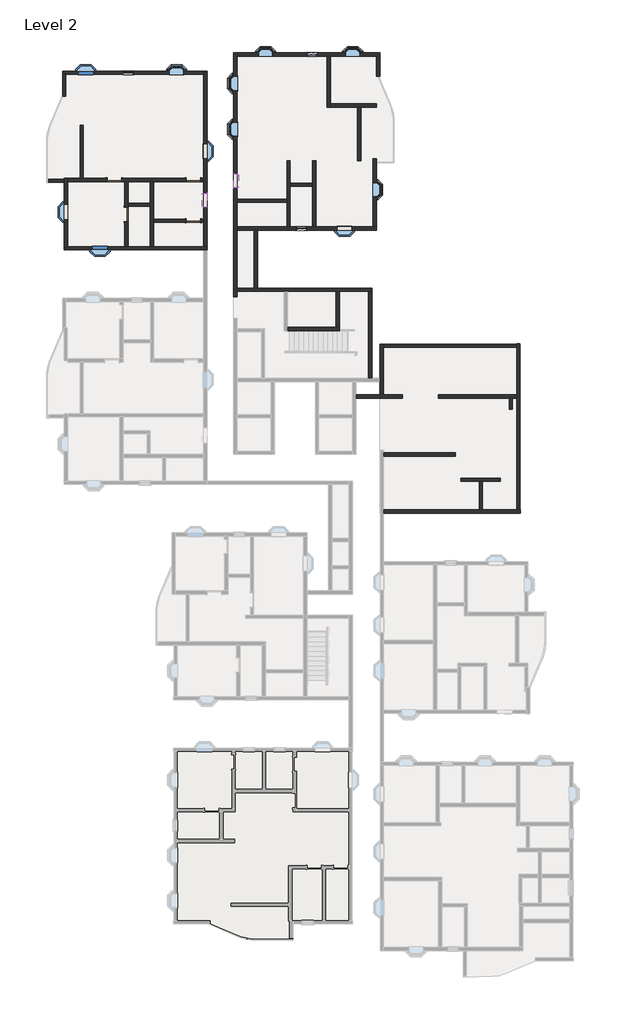
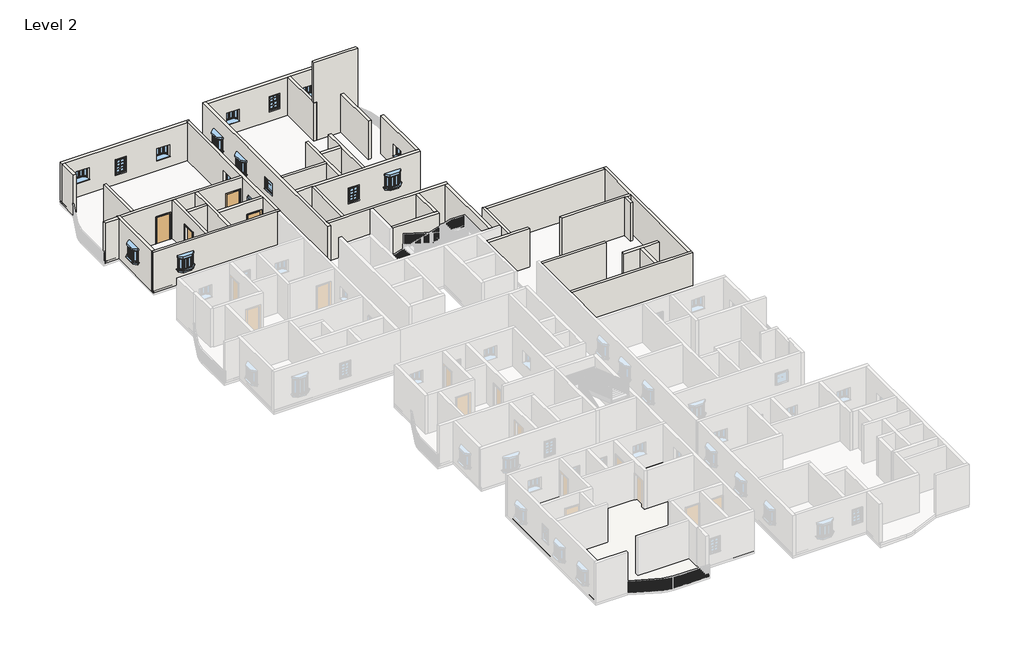
# One storey, part 4 of 14: 40 walls, 16 windows, 4 doors, 1 roof.
"""IFC4 building model written with IfcOpenShell, lengths in millimetres."""

from ifc_helpers import new_model, si_unit, point, frame, frame_2d, origin, place, context, project, spatial, polyline, circle_curve, trimmed, segment, composite_curve, outline, extrude, faceted_brep, transform, mapped, element, save
from components import door_719f80de, window_910x910mm_67ef725a, window_8debb0fa, windows_sgl_w_glazing_bars_910x910mm_256712d0

model = new_model("IFC4")

# Units and contexts
model_context = context("Model", 3, world=origin())
ifc_project = project(units=[si_unit("LENGTHUNIT", "METRE", prefix="MILLI")], contexts=[model_context])

# Site, building, storey
site = spatial("IfcSite", under=ifc_project)
building = spatial("IfcBuilding", under=site)
storey = spatial("IfcBuildingStorey", under=building, Name="Level 2", Elevation=3048.0)

# Doors
placement = place(None, origin())
door_shape = door_719f80de(model_context)
element("IfcDoor", 1, ObjectType="Single-Flush : 36\" x 84\"", at=placement, inside=storey, context=model_context, shape_type="MappedRepresentation", body=[
    mapped(door_shape, transform((-16068.1391351, 22048.4083494, 3048.0), x_axis=(1.0, 0.0, 0.0), y_axis=(0.0, 1.0, 0.0), z_axis=(0.0, 0.0, 1.0))),
])
element("IfcDoor", 2, ObjectType="Single-Flush : 36\" x 84\"", at=placement, inside=storey, context=model_context, shape_type="MappedRepresentation", body=[
    mapped(door_shape, transform((-15306.1391351, 19864.0083494, 3048.0), x_axis=(0.0, 1.0, 0.0), y_axis=(-1.0, 0.0, 0.0), z_axis=(0.0, 0.0, 1.0))),
])
element("IfcDoor", 3, ObjectType="Single-Flush : 36\" x 84\"", at=placement, inside=storey, context=model_context, shape_type="MappedRepresentation", body=[
    mapped(door_shape, transform((-11057.9891351, 19470.3083494, 3048.0), x_axis=(1.0, 0.0, 0.0), y_axis=(0.0, 1.0, 0.0), z_axis=(0.0, 0.0, 1.0))),
])
element("IfcDoor", 4, ObjectType="Single-Flush : 36\" x 84\"", at=placement, inside=storey, context=model_context, shape_type="MappedRepresentation", body=[
    mapped(door_shape, transform((-11057.9891351, 22048.4083494, 3048.0), x_axis=(1.0, 0.0, 0.0), y_axis=(0.0, 1.0, 0.0), z_axis=(0.0, 0.0, 1.0))),
])

# Roof
element("IfcRoof", 5, ObjectType="Generic - 12\"", at=placement, inside=storey, context=model_context, shape_type="SweptSolid", body=[
    extrude(outline(composite_curve([segment(polyline([(-10024.8708389, -25100.3416506), (-12290.487215, -25100.3416506), (-12290.487215, -13962.4416506), (-986.8891351, -13962.4416506), (-986.8891351, -25100.3416506), (-4746.0891351, -25100.3416506), (-4746.0891351, -26090.9416506), (-7315.6413127, -26090.9416506)]), True, "CONTINUOUS"), segment(trimmed(circle_curve(frame_2d((-7315.6413127, -24160.5416506)), 1930.4), [point((-7315.6413127, -26090.9416506))], [point((-8075.5356374, -25935.0851906))], False, "CARTESIAN"), True, "CONTINUOUS"), segment(polyline([(-8075.5356374, -25935.0851906), (-10024.8708389, -25100.3416506)]), True, "CONTINUOUS")], self_intersect=False)), frame((0.0, 0.0, 3048.0), z_axis=(0.0, 0.0, 1.0), x_axis=(1.0, 0.0, 0.0)), (0.0, 0.0, 1.0), 152.4),
])

# Walls
element("IfcWall", 6, ObjectType="4.5\" p", at=placement, inside=storey, context=model_context, shape_type="Brep", body=[
    faceted_brep([(-10600.7891351, 21946.8083494, 5181.6), (-10600.7891351, 21946.8083494, 3048.0), (-10397.5891351, 21946.8083494, 3048.0), (-10397.5891351, 21946.8083494, 6096.0), (-13578.9391351, 21946.8083494, 6096.0), (-13782.1391351, 21946.8083494, 6096.0), (-15204.5391351, 21946.8083494, 6096.0), (-15407.7391351, 21946.8083494, 6096.0), (-19033.5891351, 21946.8083494, 6096.0), (-19033.5891351, 21946.8083494, 3048.0), (-16525.3391351, 21946.8083494, 3048.0), (-16525.3391351, 21946.8083494, 5181.6), (-15610.9391351, 21946.8083494, 5181.6), (-15610.9391351, 21946.8083494, 3048.0), (-15407.7391351, 21946.8083494, 3048.0), (-15204.5391351, 21946.8083494, 3048.0), (-13782.1391351, 21946.8083494, 3048.0), (-13578.9391351, 21946.8083494, 3048.0), (-11515.1891351, 21946.8083494, 3048.0), (-11515.1891351, 21946.8083494, 5181.6), (-10397.5891351, 22150.0083494, 3048.0), (-10600.7891351, 22150.0083494, 3048.0), (-10600.7891351, 22150.0083494, 5181.6), (-11515.1891351, 22150.0083494, 5181.6), (-11515.1891351, 22150.0083494, 3048.0), (-15610.9391351, 22150.0083494, 3048.0), (-15610.9391351, 22150.0083494, 5181.6), (-16525.3391351, 22150.0083494, 5181.6), (-16525.3391351, 22150.0083494, 3048.0), (-18042.9891351, 22150.0083494, 3048.0), (-18246.1891351, 22150.0083494, 3048.0), (-19033.5891351, 22150.0083494, 3048.0), (-19033.5891351, 22150.0083494, 6096.0), (-18246.1891351, 22150.0083494, 6096.0), (-18042.9891351, 22150.0083494, 6096.0), (-10397.5891351, 22150.0083494, 6096.0)], [[[0, 1, 2, 3, 4, 5, 6, 7, 8, 9, 10, 11, 12, 13, 14, 15, 16, 17, 18, 19]], [[20, 21, 22, 23, 24, 25, 26, 27, 28, 29, 30, 31, 32, 33, 34, 35]], [[10, 9, 31, 30, 29, 28]], [[2, 1, 21, 20]], [[18, 17, 16, 15, 14, 13, 25, 24]], [[8, 7, 6, 5, 4, 3, 35, 34, 33, 32]], [[9, 8, 32, 31]], [[3, 2, 20, 35]], [[26, 25, 13, 12]], [[27, 26, 12, 11]], [[28, 27, 11, 10]], [[22, 21, 1, 0]], [[23, 22, 0, 19]], [[24, 23, 19, 18]]]),
])
element("IfcWall", 7, ObjectType="4.5\" p", at=placement, inside=storey, context=model_context, shape_type="Brep", body=[
    faceted_brep([(-15407.7391351, 21946.8083494, 3048.0), (-15407.7391351, 20321.2083494, 3048.0), (-15407.7391351, 20321.2083494, 5181.6), (-15407.7391351, 19406.8083494, 5181.6), (-15407.7391351, 19406.8083494, 3048.0), (-15407.7391351, 17812.9583494, 3048.0), (-15407.7391351, 17812.9583494, 6096.0), (-15407.7391351, 21946.8083494, 6096.0), (-15204.5391351, 20321.2083494, 5181.6), (-15204.5391351, 20321.2083494, 3048.0), (-15204.5391351, 20372.0083494, 3048.0), (-15204.5391351, 20575.2083494, 3048.0), (-15204.5391351, 21946.8083494, 3048.0), (-15204.5391351, 21946.8083494, 6096.0), (-15204.5391351, 20575.2083494, 6096.0), (-15204.5391351, 20372.0083494, 6096.0), (-15204.5391351, 17812.9583494, 6096.0), (-15204.5391351, 17812.9583494, 3048.0), (-15204.5391351, 19406.8083494, 3048.0), (-15204.5391351, 19406.8083494, 5181.6)], [[[0, 1, 2, 3, 4, 5, 6, 7]], [[8, 9, 10, 11, 12, 13, 14, 15, 16, 17, 18, 19]], [[18, 17, 5, 4]], [[12, 11, 10, 9, 1, 0]], [[7, 6, 16, 15, 14, 13]], [[6, 5, 17, 16]], [[0, 7, 13, 12]], [[2, 1, 9, 8]], [[3, 2, 8, 19]], [[4, 3, 19, 18]]]),
])
element("IfcWall", 8, ObjectType="4.5\" p", at=placement, inside=storey, context=model_context, shape_type="Brep", body=[
    faceted_brep([(-13782.1391351, 21946.8083494, 3048.0), (-13782.1391351, 20575.2083494, 3048.0), (-13782.1391351, 20372.0083494, 3048.0), (-13782.1391351, 17812.9583494, 3048.0), (-13782.1391351, 17812.9583494, 6096.0), (-13782.1391351, 20372.0083494, 6096.0), (-13782.1391351, 20575.2083494, 6096.0), (-13782.1391351, 21946.8083494, 6096.0), (-13578.9391351, 21946.8083494, 3048.0), (-13578.9391351, 21946.8083494, 6096.0), (-13578.9391351, 19571.9083494, 6096.0), (-13578.9391351, 19368.7083494, 6096.0), (-13578.9391351, 17812.9583494, 6096.0), (-13578.9391351, 17812.9583494, 3048.0), (-13578.9391351, 19368.7083494, 3048.0), (-13578.9391351, 19571.9083494, 3048.0)], [[[0, 1, 2, 3, 4, 5, 6, 7]], [[8, 9, 10, 11, 12, 13, 14, 15]], [[3, 2, 1, 0, 8, 15, 14, 13]], [[7, 6, 5, 4, 12, 11, 10, 9]], [[4, 3, 13, 12]], [[0, 7, 9, 8]]]),
])
element("IfcWall", 9, ObjectType="4.5\" p", at=placement, inside=storey, context=model_context, shape_type="SweptSolid", body=[
    extrude(outline(polyline([(-13782.1391351, 20372.0083494), (-15204.5391351, 20372.0083494), (-15204.5391351, 20575.2083494), (-13782.1391351, 20575.2083494), (-13782.1391351, 20372.0083494)])), frame((0.0, 0.0, 3048.0), z_axis=(0.0, 0.0, 1.0), x_axis=(1.0, 0.0, 0.0)), (0.0, 0.0, 1.0), 3048.0),
])
element("IfcWall", 10, ObjectType="4.5\" p", at=placement, inside=storey, context=model_context, shape_type="SweptSolid", body=[
    extrude(outline(polyline([(5181.6, -10600.7891351), (3048.0, -10600.7891351), (3048.0, -10397.5891351), (6096.0, -10397.5891351), (6096.0, -13578.9391351), (3048.0, -13578.9391351), (3048.0, -11515.1891351), (5181.6, -11515.1891351), (5181.6, -10600.7891351)])), frame((0.0, 19368.7083494, 0.0), z_axis=(0.0, 1.0, 0.0), x_axis=(0.0, 0.0, 1.0)), (0.0, 0.0, 1.0), 203.2),
])
element("IfcWall", 11, ObjectType="4.5\" p", at=placement, inside=storey, context=model_context, shape_type="SweptSolid", body=[
    extrude(outline(polyline([(-18246.1891351, 22150.0083494), (-18246.1891351, 25515.5083494), (-18042.9891351, 25515.5083494), (-18042.9891351, 22150.0083494), (-18246.1891351, 22150.0083494)])), frame((0.0, 0.0, 3048.0), z_axis=(0.0, 0.0, 1.0), x_axis=(1.0, 0.0, 0.0)), (0.0, 0.0, 1.0), 3048.0),
])
element("IfcWall", 12, ObjectType="4.5\" p", at=placement, inside=storey, context=model_context, shape_type="SweptSolid", body=[
    extrude(outline(polyline([(-6993.9891351, 18875.1215905), (-6993.9891351, 15192.1215905), (-7197.1891351, 15192.1215905), (-7197.1891351, 18875.1215905), (-6993.9891351, 18875.1215905)])), frame((0.0, 0.0, 3048.0), z_axis=(0.0, 0.0, 1.0), x_axis=(1.0, 0.0, 0.0)), (0.0, 0.0, 1.0), 3048.0),
])
element("IfcWall", 13, ObjectType="4.5\" p", at=placement, inside=storey, context=model_context, shape_type="Brep", body=[
    faceted_brep([(-8289.3891351, 18875.1215905, 3048.0), (-7197.1891351, 18875.1215905, 3048.0), (-6993.9891351, 18875.1215905, 3048.0), (562.5108649, 18875.1215905, 3048.0), (562.5108649, 18875.1215905, 6096.0), (-6993.9891351, 18875.1215905, 6096.0), (-7197.1891351, 18875.1215905, 6096.0), (-8289.3891351, 18875.1215905, 6096.0), (-1017.6641351, 18875.1215905, 5158.0), (-1017.6641351, 18875.1215905, 4248.0), (-1927.6641351, 18875.1215905, 4248.0), (-1927.6641351, 18875.1215905, 5158.0), (-3876.1391351, 18875.1215905, 5029.2), (-3876.1391351, 18875.1215905, 3962.4), (-4536.5391351, 18875.1215905, 3962.4), (-4536.5391351, 18875.1215905, 5029.2), (-8289.3891351, 19078.3215905, 3048.0), (-8289.3891351, 19078.3215905, 6096.0), (-5120.7391351, 19078.3215905, 6096.0), (-4917.5391351, 19078.3215905, 6096.0), (-3495.1391351, 19078.3215905, 6096.0), (-3291.9391351, 19078.3215905, 6096.0), (346.6108649, 19078.3215905, 6096.0), (549.8108649, 19078.3215905, 6096.0), (562.5108649, 19078.3215905, 6096.0), (562.5108649, 19078.3215905, 3048.0), (549.8108649, 19078.3215905, 3048.0), (346.6108649, 19078.3215905, 3048.0), (-3291.9391351, 19078.3215905, 3048.0), (-3495.1391351, 19078.3215905, 3048.0), (-4917.5391351, 19078.3215905, 3048.0), (-5120.7391351, 19078.3215905, 3048.0), (-1017.6641351, 19078.3215905, 5158.0), (-1927.6641351, 19078.3215905, 5158.0), (-1927.6641351, 19078.3215905, 4248.0), (-1017.6641351, 19078.3215905, 4248.0), (-3876.1391351, 19078.3215905, 5029.2), (-4536.5391351, 19078.3215905, 5029.2), (-4536.5391351, 19078.3215905, 3962.4), (-3876.1391351, 19078.3215905, 3962.4)], [[[0, 1, 2, 3, 4, 5, 6, 7], [8, 9, 10, 11], [12, 13, 14, 15]], [[16, 17, 18, 19, 20, 21, 22, 23, 24, 25, 26, 27, 28, 29, 30, 31], [32, 33, 34, 35], [36, 37, 38, 39]], [[3, 2, 1, 0, 16, 31, 30, 29, 28, 27, 26, 25]], [[4, 3, 25, 24]], [[7, 6, 5, 4, 24, 23, 22, 21, 20, 19, 18, 17]], [[0, 7, 17, 16]], [[9, 8, 32, 35]], [[10, 9, 35, 34]], [[11, 10, 34, 33]], [[8, 11, 33, 32]], [[13, 12, 36, 39]], [[14, 13, 39, 38]], [[15, 14, 38, 37]], [[12, 15, 37, 36]]]),
])
element("IfcWall", 14, ObjectType="4.5\" p", at=placement, inside=storey, context=model_context, shape_type="SweptSolid", body=[
    extrude(outline(polyline([(19078.3215905, 3048.0), (19078.3215905, 6096.0), (23396.3215905, 6096.0), (23396.3215905, 3048.0), (19078.3215905, 3048.0)]), holes=[polyline([(21882.8215905, 4872.4), (20972.8215905, 4872.4), (20972.8215905, 3962.4), (21882.8215905, 3962.4), (21882.8215905, 4872.4)])]), frame((346.6108649, 0.0, 0.0), z_axis=(1.0, 0.0, 0.0), x_axis=(0.0, 1.0, 0.0)), (0.0, 0.0, 1.0), 203.2),
])
element("IfcWall", 15, ObjectType="4.5\" p", at=placement, inside=storey, context=model_context, shape_type="SweptSolid", body=[
    extrude(outline(polyline([(-5120.7391351, 20634.0715905), (-8289.3891351, 20634.0715905), (-8289.3891351, 20837.2715905), (-5120.7391351, 20837.2715905), (-5120.7391351, 20634.0715905)])), frame((0.0, 0.0, 3048.0), z_axis=(0.0, 0.0, 1.0), x_axis=(1.0, 0.0, 0.0)), (0.0, 0.0, 1.0), 3048.0),
])
element("IfcWall", 16, ObjectType="4.5\" p", at=placement, inside=storey, context=model_context, shape_type="Brep", body=[
    faceted_brep([(-5120.7391351, 23256.6215905, 3048.0), (-5120.7391351, 20837.2715905, 3048.0), (-5120.7391351, 20634.0715905, 3048.0), (-5120.7391351, 19078.3215905, 3048.0), (-5120.7391351, 19078.3215905, 6096.0), (-5120.7391351, 20634.0715905, 6096.0), (-5120.7391351, 20837.2715905, 6096.0), (-5120.7391351, 23256.6215905, 6096.0), (-4917.5391351, 23256.6215905, 3048.0), (-4917.5391351, 23256.6215905, 6096.0), (-4917.5391351, 21853.2715905, 6096.0), (-4917.5391351, 21650.0715905, 6096.0), (-4917.5391351, 19078.3215905, 6096.0), (-4917.5391351, 19078.3215905, 3048.0), (-4917.5391351, 21650.0715905, 3048.0), (-4917.5391351, 21853.2715905, 3048.0)], [[[0, 1, 2, 3, 4, 5, 6, 7]], [[8, 9, 10, 11, 12, 13, 14, 15]], [[3, 2, 1, 0, 8, 15, 14, 13]], [[7, 6, 5, 4, 12, 11, 10, 9]], [[0, 7, 9, 8]], [[4, 3, 13, 12]]]),
])
element("IfcWall", 17, ObjectType="4.5\" p", at=placement, inside=storey, context=model_context, shape_type="Brep", body=[
    faceted_brep([(-3495.1391351, 23256.6215905, 3048.0), (-3495.1391351, 21853.2715905, 3048.0), (-3495.1391351, 21650.0715905, 3048.0), (-3495.1391351, 19078.3215905, 3048.0), (-3495.1391351, 19078.3215905, 6096.0), (-3495.1391351, 21650.0715905, 6096.0), (-3495.1391351, 21853.2715905, 6096.0), (-3495.1391351, 23256.6215905, 6096.0), (-3291.9391351, 23256.6215905, 3048.0), (-3291.9391351, 23256.6215905, 6096.0), (-3291.9391351, 19078.3215905, 6096.0), (-3291.9391351, 19078.3215905, 3048.0)], [[[0, 1, 2, 3, 4, 5, 6, 7]], [[8, 9, 10, 11]], [[3, 2, 1, 0, 8, 11]], [[7, 6, 5, 4, 10, 9]], [[0, 7, 9, 8]], [[4, 3, 11, 10]]]),
])
element("IfcWall", 18, ObjectType="4.5\" p", at=placement, inside=storey, context=model_context, shape_type="SweptSolid", body=[
    extrude(outline(polyline([(-3495.1391351, 21650.0715905), (-4917.5391351, 21650.0715905), (-4917.5391351, 21853.2715905), (-3495.1391351, 21853.2715905), (-3495.1391351, 21650.0715905)])), frame((0.0, 0.0, 3048.0), z_axis=(0.0, 0.0, 1.0), x_axis=(1.0, 0.0, 0.0)), (0.0, 0.0, 1.0), 3048.0),
])
element("IfcWall", 19, ObjectType="4.5\" p", at=placement, inside=storey, context=model_context, shape_type="SweptSolid", body=[
    extrude(outline(polyline([(-1799.6891351, 14988.9215905), (-1799.6891351, 12709.2715905), (-2002.8891351, 12709.2715905), (-2002.8891351, 14988.9215905), (-1799.6891351, 14988.9215905)])), frame((0.0, 0.0, 3048.0), z_axis=(0.0, 0.0, 1.0), x_axis=(1.0, 0.0, 0.0)), (0.0, 0.0, 1.0), 3048.0),
])
element("IfcWall", 20, ObjectType="4.5\" p", at=placement, inside=storey, context=model_context, shape_type="Brep", body=[
    faceted_brep([(-5095.3391351, 12506.0715905, 3048.0), (-1786.9891351, 12506.0715905, 3048.0), (-1786.9891351, 12506.0715905, 6096.0), (-5095.3391351, 12506.0715905, 6096.0), (-5095.3391351, 12709.2715905, 3048.0), (-5095.3391351, 12709.2715905, 6096.0), (-2002.8891351, 12709.2715905, 6096.0), (-1799.6891351, 12709.2715905, 6096.0), (-1786.9891351, 12709.2715905, 6096.0), (-1786.9891351, 12709.2715905, 3048.0), (-1799.6891351, 12709.2715905, 3048.0), (-2002.8891351, 12709.2715905, 3048.0)], [[[0, 1, 2, 3]], [[4, 5, 6, 7, 8, 9, 10, 11]], [[1, 0, 4, 11, 10, 9]], [[2, 1, 9, 8]], [[3, 2, 8, 7, 6, 5]], [[0, 3, 5, 4]]]),
])
element("IfcWall", 21, ObjectType="4.5\" p", at=placement, inside=storey, context=model_context, shape_type="Brep", body=[
    faceted_brep([(-745.5891351, 8223.6457306, 3048.0), (2209.4205024, 8223.6457306, 3048.0), (2209.4205024, 8223.6457306, 6096.0), (-745.5891351, 8223.6457306, 6096.0), (-745.5891351, 8426.8457306, 3048.0), (-745.5891351, 8426.8457306, 6096.0), (793.5880523, 8426.8457306, 6096.0), (996.7880523, 8426.8457306, 6096.0), (2209.4205024, 8426.8457306, 6096.0), (2209.4205024, 8426.8457306, 3048.0), (996.7880523, 8426.8457306, 3048.0), (793.5880523, 8426.8457306, 3048.0)], [[[0, 1, 2, 3]], [[4, 5, 6, 7, 8, 9, 10, 11]], [[1, 0, 4, 11, 10, 9]], [[2, 1, 9, 8]], [[3, 2, 8, 7, 6, 5]], [[0, 3, 5, 4]]]),
])
element("IfcWall", 22, ObjectType="4.5\" p", at=placement, inside=storey, context=model_context, shape_type="Brep", body=[
    faceted_brep([(996.7880523, 8426.8457306, 3048.0), (996.7880523, 11443.0957306, 3048.0), (996.7880523, 11646.2957306, 3048.0), (996.7880523, 11646.2957306, 6096.0), (996.7880523, 11443.0957306, 6096.0), (996.7880523, 8426.8457306, 6096.0), (793.5880523, 8426.8457306, 3048.0), (793.5880523, 8426.8457306, 6096.0), (793.5880523, 9275.2949943, 6096.0), (793.5880523, 9478.4949943, 6096.0), (793.5880523, 11646.2957306, 6096.0), (793.5880523, 11646.2957306, 3048.0), (793.5880523, 9478.4949943, 3048.0), (793.5880523, 9275.2949943, 3048.0)], [[[0, 1, 2, 3, 4, 5]], [[6, 7, 8, 9, 10, 11, 12, 13]], [[2, 1, 0, 6, 13, 12, 11]], [[5, 4, 3, 10, 9, 8, 7]], [[0, 5, 7, 6]], [[3, 2, 11, 10]]]),
])
element("IfcWall", 23, ObjectType="4.5\" p", at=placement, inside=storey, context=model_context, shape_type="Brep", body=[
    faceted_brep([(9461.3380523, 8426.8457306, 3048.0), (4492.3034266, 8426.8457306, 3048.0), (4492.3034266, 8426.8457306, 6096.0), (9461.3380523, 8426.8457306, 6096.0), (9461.3380523, 8223.6457306, 3048.0), (9461.3380523, 8223.6457306, 6096.0), (9181.9380523, 8223.6457306, 6096.0), (8978.7380523, 8223.6457306, 6096.0), (4492.3034266, 8223.6457306, 6096.0), (4492.3034266, 8223.6457306, 3048.0), (8978.7380523, 8223.6457306, 3048.0), (9181.9380523, 8223.6457306, 3048.0)], [[[0, 1, 2, 3]], [[4, 5, 6, 7, 8, 9, 10, 11]], [[1, 0, 4, 11, 10, 9]], [[2, 1, 9, 8]], [[3, 2, 8, 7, 6, 5]], [[0, 3, 5, 4]]]),
])
element("IfcWall", 24, ObjectType="4.5\" p", at=placement, inside=storey, context=model_context, shape_type="Brep", body=[
    faceted_brep([(1007.0108649, 940.1957306, 3048.0), (9677.2380523, 940.1957306, 3048.0), (9677.2380523, 940.1957306, 6096.0), (1007.0108649, 940.1957306, 6096.0), (1007.0108649, 1143.3957306, 3048.0), (1007.0108649, 1143.3957306, 6096.0), (7073.7380523, 1143.3957306, 6096.0), (7276.9380523, 1143.3957306, 6096.0), (9461.3380523, 1143.3957306, 6096.0), (9664.5380523, 1143.3957306, 6096.0), (9677.2380523, 1143.3957306, 6096.0), (9677.2380523, 1143.3957306, 3048.0), (9664.5380523, 1143.3957306, 3048.0), (9461.3380523, 1143.3957306, 3048.0), (7276.9380523, 1143.3957306, 3048.0), (7073.7380523, 1143.3957306, 3048.0)], [[[0, 1, 2, 3]], [[4, 5, 6, 7, 8, 9, 10, 11, 12, 13, 14, 15]], [[1, 0, 4, 15, 14, 13, 12, 11]], [[2, 1, 11, 10]], [[3, 2, 10, 9, 8, 7, 6, 5]], [[0, 3, 5, 4]]]),
])
element("IfcWall", 25, ObjectType="4.5\" p", at=placement, inside=storey, context=model_context, shape_type="Brep", body=[
    faceted_brep([(9664.5380523, 1143.3957306, 3048.0), (9664.5380523, 11658.9957306, 3048.0), (9664.5380523, 11658.9957306, 6096.0), (9664.5380523, 1143.3957306, 6096.0), (9461.3380523, 1143.3957306, 3048.0), (9461.3380523, 1143.3957306, 6096.0), (9461.3380523, 8223.6457306, 6096.0), (9461.3380523, 8426.8457306, 6096.0), (9461.3380523, 11443.0957306, 6096.0), (9461.3380523, 11646.2957306, 6096.0), (9461.3380523, 11658.9957306, 6096.0), (9461.3380523, 11658.9957306, 3048.0), (9461.3380523, 11646.2957306, 3048.0), (9461.3380523, 11443.0957306, 3048.0), (9461.3380523, 8426.8457306, 3048.0), (9461.3380523, 8223.6457306, 3048.0)], [[[0, 1, 2, 3]], [[4, 5, 6, 7, 8, 9, 10, 11, 12, 13, 14, 15]], [[1, 0, 4, 15, 14, 13, 12, 11]], [[2, 1, 11, 10]], [[3, 2, 10, 9, 8, 7, 6, 5]], [[0, 3, 5, 4]]]),
])
element("IfcWall", 26, ObjectType="4.5\" p", at=placement, inside=storey, context=model_context, shape_type="SweptSolid", body=[
    extrude(outline(polyline([(-643.9891351, 23256.6215905), (-643.9891351, 26659.3286213), (-440.7891351, 26659.3286213), (-440.7891351, 23256.6215905), (-643.9891351, 23256.6215905)])), frame((0.0, 0.0, 3048.0), z_axis=(0.0, 0.0, 1.0), x_axis=(1.0, 0.0, 0.0)), (0.0, 0.0, 1.0), 3048.0),
])
element("IfcWall", 27, ObjectType="4.5\" p", at=placement, inside=storey, context=model_context, shape_type="Brep", body=[
    faceted_brep([(-2568.0391351, 29898.7215905, 3048.0), (-2568.0391351, 26659.3286213, 3048.0), (-2568.0391351, 26659.3286213, 6096.0), (-2568.0391351, 26862.5286213, 6096.0), (-2568.0391351, 29898.7215905, 6096.0), (-2364.8391351, 29898.7215905, 3048.0), (-2364.8391351, 29898.7215905, 6096.0), (-2364.8391351, 26862.5286213, 6096.0), (-2364.8391351, 26659.3286213, 6096.0), (-2364.8391351, 26659.3286213, 3048.0), (-2364.8391351, 26862.5286213, 3048.0)], [[[0, 1, 2, 3, 4]], [[5, 6, 7, 8, 9, 10]], [[1, 0, 5, 10, 9]], [[4, 3, 2, 8, 7, 6]], [[2, 1, 9, 8]], [[0, 4, 6, 5]]]),
])
element("IfcWall", 28, ObjectType="4.5\" p", at=placement, inside=storey, context=model_context, shape_type="Brep", body=[
    faceted_brep([(-2364.8391351, 26659.3286213, 3048.0), (-643.9891351, 26659.3286213, 3048.0), (-440.7891351, 26659.3286213, 3048.0), (562.5108649, 26659.3286213, 3048.0), (562.5108649, 26659.3286213, 9144.0), (-440.7891351, 26659.3286213, 9144.0), (-643.9891351, 26659.3286213, 9144.0), (-2568.0391351, 26659.3286213, 9144.0), (-2568.0391351, 26659.3286213, 6096.0), (-2364.8391351, 26659.3286213, 6096.0), (-2364.8391351, 26862.5286213, 3048.0), (-2364.8391351, 26862.5286213, 6096.0), (-2568.0391351, 26862.5286213, 6096.0), (-2568.0391351, 26862.5286213, 9144.0), (-2364.8391351, 26862.5286213, 9144.0), (562.5108649, 26862.5286213, 9144.0), (562.5108649, 26862.5286213, 3048.0)], [[[0, 1, 2, 3, 4, 5, 6, 7, 8, 9]], [[10, 11, 12, 13, 14, 15, 16]], [[3, 2, 1, 0, 10, 16]], [[4, 3, 16, 15]], [[7, 6, 5, 4, 15, 14, 13]], [[8, 12, 11, 9]], [[0, 9, 11, 10]], [[8, 7, 13, 12]]]),
])
element("IfcWall", 29, ObjectType="4.5\" p", at=placement, inside=storey, context=model_context, shape_type="SweptSolid", body=[
    extrude(outline(polyline([(-2568.0391351, 26862.5286213), (-2568.0391351, 29898.7215905), (-2364.8391351, 29898.7215905), (-2364.8391351, 26862.5286213), (-2568.0391351, 26862.5286213)])), frame((0.0, 0.0, 3048.0), z_axis=(0.0, 0.0, 1.0), x_axis=(1.0, 0.0, 0.0)), (0.0, 0.0, 1.0), 3048.0),
])
element("IfcWall", 30, ObjectType="4.5\" p", at=placement, inside=storey, context=model_context, shape_type="SweptSolid", body=[
    extrude(outline(polyline([(765.7108649, 29898.7215905), (765.7108649, 28631.1875845), (562.5108649, 28631.1875845), (562.5108649, 29898.7215905), (765.7108649, 29898.7215905)])), frame((0.0, 0.0, 3048.0), z_axis=(0.0, 0.0, 1.0), x_axis=(1.0, 0.0, 0.0)), (0.0, 0.0, 1.0), 3048.0),
])
element("IfcWall", 31, ObjectType="9\" w", at=placement, inside=storey, context=model_context, shape_type="Brep", body=[
    faceted_brep([(-10181.6891351, 17812.9583494, 3048.0), (-10194.3891351, 17812.9583494, 3048.0), (-10397.5891351, 17812.9583494, 3048.0), (-13578.9391351, 17812.9583494, 3048.0), (-13782.1391351, 17812.9583494, 3048.0), (-15204.5391351, 17812.9583494, 3048.0), (-15407.7391351, 17812.9583494, 3048.0), (-19033.5891351, 17812.9583494, 3048.0), (-19236.7891351, 17812.9583494, 3048.0), (-19249.4891351, 17812.9583494, 3048.0), (-19249.4891351, 17812.9583494, 6096.0), (-19236.7891351, 17812.9583494, 6096.0), (-19033.5891351, 17812.9583494, 6096.0), (-15407.7391351, 17812.9583494, 6096.0), (-15204.5391351, 17812.9583494, 6096.0), (-13782.1391351, 17812.9583494, 6096.0), (-13578.9391351, 17812.9583494, 6096.0), (-10397.5891351, 17812.9583494, 6096.0), (-10194.3891351, 17812.9583494, 6096.0), (-10181.6891351, 17812.9583494, 6096.0), (-16527.5391351, 17812.9583494, 5158.0), (-17437.5391351, 17812.9583494, 5158.0), (-17437.5391351, 17812.9583494, 4248.0), (-16527.5391351, 17812.9583494, 4248.0), (-10181.6891351, 17609.7583494, 3048.0), (-10181.6891351, 17609.7583494, 6096.0), (-19249.4891351, 17609.7583494, 6096.0), (-19249.4891351, 17609.7583494, 3048.0), (-16527.5391351, 17609.7583494, 5158.0), (-16527.5391351, 17609.7583494, 4248.0), (-17437.5391351, 17609.7583494, 4248.0), (-17437.5391351, 17609.7583494, 5158.0)], [[[0, 1, 2, 3, 4, 5, 6, 7, 8, 9, 10, 11, 12, 13, 14, 15, 16, 17, 18, 19], [20, 21, 22, 23]], [[24, 25, 26, 27], [28, 29, 30, 31]], [[9, 8, 7, 6, 5, 4, 3, 2, 1, 0, 24, 27]], [[10, 9, 27, 26]], [[19, 18, 17, 16, 15, 14, 13, 12, 11, 10, 26, 25]], [[0, 19, 25, 24]], [[29, 28, 20, 23]], [[30, 29, 23, 22]], [[31, 30, 22, 21]], [[28, 31, 21, 20]]]),
])
element("IfcWall", 32, ObjectType="9\" w", at=placement, inside=storey, context=model_context, shape_type="Brep", body=[
    faceted_brep([(-19033.5891351, 17812.9583494, 3048.0), (-19033.5891351, 21946.8083494, 3048.0), (-19033.5891351, 22150.0083494, 3048.0), (-19033.5891351, 22150.0083494, 6096.0), (-19033.5891351, 21946.8083494, 6096.0), (-19033.5891351, 17812.9583494, 6096.0), (-19033.5891351, 19555.0583494, 5158.0), (-19033.5891351, 20465.0583494, 5158.0), (-19033.5891351, 20465.0583494, 4248.0), (-19033.5891351, 19555.0583494, 4248.0), (-19236.7891351, 17812.9583494, 3048.0), (-19236.7891351, 17812.9583494, 6096.0), (-19236.7891351, 21889.6583494, 6096.0), (-19236.7891351, 22092.8583494, 6096.0), (-19236.7891351, 22150.0083494, 6096.0), (-19236.7891351, 22150.0083494, 3048.0), (-19236.7891351, 22092.8583494, 3048.0), (-19236.7891351, 21889.6583494, 3048.0), (-19236.7891351, 19555.0583494, 5158.0), (-19236.7891351, 19555.0583494, 4248.0), (-19236.7891351, 20465.0583494, 4248.0), (-19236.7891351, 20465.0583494, 5158.0)], [[[0, 1, 2, 3, 4, 5], [6, 7, 8, 9]], [[10, 11, 12, 13, 14, 15, 16, 17], [18, 19, 20, 21]], [[2, 1, 0, 10, 17, 16, 15]], [[5, 4, 3, 14, 13, 12, 11]], [[0, 5, 11, 10]], [[3, 2, 15, 14]], [[19, 18, 6, 9]], [[20, 19, 9, 8]], [[21, 20, 8, 7]], [[18, 21, 7, 6]]]),
])
element("IfcWall", 33, ObjectType="9\" w", at=placement, inside=storey, context=model_context, shape_type="Brep", body=[
    faceted_brep([(-10194.3891351, 17812.9583494, 3048.0), (-10194.3891351, 28849.2583494, 3048.0), (-10194.3891351, 28849.2583494, 6096.0), (-10194.3891351, 17812.9583494, 6096.0), (-10194.3891351, 24319.5083494, 5158.0), (-10194.3891351, 24319.5083494, 4248.0), (-10194.3891351, 23409.5083494, 4248.0), (-10194.3891351, 23409.5083494, 5158.0), (-10194.3891351, 20304.3583494, 5158.0), (-10194.3891351, 21214.3583494, 5158.0), (-10194.3891351, 21214.3583494, 4248.0), (-10194.3891351, 20304.3583494, 4248.0), (-10397.5891351, 17812.9583494, 3048.0), (-10397.5891351, 17812.9583494, 6096.0), (-10397.5891351, 19368.7083494, 6096.0), (-10397.5891351, 19571.9083494, 6096.0), (-10397.5891351, 21946.8083494, 6096.0), (-10397.5891351, 22150.0083494, 6096.0), (-10397.5891351, 28849.2583494, 6096.0), (-10397.5891351, 28849.2583494, 3048.0), (-10397.5891351, 22150.0083494, 3048.0), (-10397.5891351, 21946.8083494, 3048.0), (-10397.5891351, 19571.9083494, 3048.0), (-10397.5891351, 19368.7083494, 3048.0), (-10397.5891351, 24319.5083494, 5158.0), (-10397.5891351, 23409.5083494, 5158.0), (-10397.5891351, 23409.5083494, 4248.0), (-10397.5891351, 24319.5083494, 4248.0), (-10397.5891351, 20304.3583494, 5158.0), (-10397.5891351, 20304.3583494, 4248.0), (-10397.5891351, 21214.3583494, 4248.0), (-10397.5891351, 21214.3583494, 5158.0)], [[[0, 1, 2, 3], [4, 5, 6, 7], [8, 9, 10, 11]], [[12, 13, 14, 15, 16, 17, 18, 19, 20, 21, 22, 23], [24, 25, 26, 27], [28, 29, 30, 31]], [[1, 0, 12, 23, 22, 21, 20, 19]], [[2, 1, 19, 18]], [[3, 2, 18, 17, 16, 15, 14, 13]], [[0, 3, 13, 12]], [[5, 4, 24, 27]], [[6, 5, 27, 26]], [[7, 6, 26, 25]], [[4, 7, 25, 24]], [[29, 28, 8, 11]], [[30, 29, 11, 10]], [[31, 30, 10, 9]], [[28, 31, 9, 8]]]),
])
element("IfcWall", 34, ObjectType="9\" w", at=placement, inside=storey, context=model_context, shape_type="SweptSolid", body=[
    extrude(outline(polyline([(-19236.7891351, 21889.6583494), (-20240.0891351, 21889.6583494), (-20240.0891351, 22092.8583494), (-19236.7891351, 22092.8583494), (-19236.7891351, 21889.6583494)])), frame((0.0, 0.0, 3048.0), z_axis=(0.0, 0.0, 1.0), x_axis=(1.0, 0.0, 0.0)), (0.0, 0.0, 1.0), 3048.0),
])
element("IfcWall", 35, ObjectType="9\" w", at=placement, inside=storey, context=model_context, shape_type="Brep", body=[
    faceted_brep([(-8492.5891351, 30114.6215905, 3048.0), (-8492.5891351, 14654.9471999, 3048.0), (-8492.5891351, 14654.9471999, 6096.0), (-8492.5891351, 30114.6215905, 6096.0), (-8492.5891351, 27703.9922564, 4872.4), (-8492.5891351, 27703.9922564, 3962.4), (-8492.5891351, 28613.9922564, 3962.4), (-8492.5891351, 28613.9922564, 4872.4), (-8492.5891351, 24808.3922564, 4872.4), (-8492.5891351, 24808.3922564, 3962.4), (-8492.5891351, 25718.3922564, 3962.4), (-8492.5891351, 25718.3922564, 4872.4), (-8492.5891351, 22451.1465905, 5158.0), (-8492.5891351, 21541.1465905, 5158.0), (-8492.5891351, 21541.1465905, 4248.0), (-8492.5891351, 22451.1465905, 4248.0), (-8289.3891351, 30114.6215905, 3048.0), (-8289.3891351, 30114.6215905, 6096.0), (-8289.3891351, 30101.9215905, 6096.0), (-8289.3891351, 29898.7215905, 6096.0), (-8289.3891351, 20837.2715905, 6096.0), (-8289.3891351, 20634.0715905, 6096.0), (-8289.3891351, 19078.3215905, 6096.0), (-8289.3891351, 18875.1215905, 6096.0), (-8289.3891351, 15192.1215905, 6096.0), (-8289.3891351, 14988.9215905, 6096.0), (-8289.3891351, 14654.9471999, 6096.0), (-8289.3891351, 14654.9471999, 3048.0), (-8289.3891351, 14988.9215905, 3048.0), (-8289.3891351, 15192.1215905, 3048.0), (-8289.3891351, 18875.1215905, 3048.0), (-8289.3891351, 19078.3215905, 3048.0), (-8289.3891351, 20634.0715905, 3048.0), (-8289.3891351, 20837.2715905, 3048.0), (-8289.3891351, 29898.7215905, 3048.0), (-8289.3891351, 30101.9215905, 3048.0), (-8289.3891351, 27703.9922564, 4872.4), (-8289.3891351, 28613.9922564, 4872.4), (-8289.3891351, 28613.9922564, 3962.4), (-8289.3891351, 27703.9922564, 3962.4), (-8289.3891351, 24808.3922564, 4872.4), (-8289.3891351, 25718.3922564, 4872.4), (-8289.3891351, 25718.3922564, 3962.4), (-8289.3891351, 24808.3922564, 3962.4), (-8289.3891351, 22451.1465905, 5158.0), (-8289.3891351, 22451.1465905, 4248.0), (-8289.3891351, 21541.1465905, 4248.0), (-8289.3891351, 21541.1465905, 5158.0)], [[[0, 1, 2, 3], [4, 5, 6, 7], [8, 9, 10, 11], [12, 13, 14, 15]], [[16, 17, 18, 19, 20, 21, 22, 23, 24, 25, 26, 27, 28, 29, 30, 31, 32, 33, 34, 35], [36, 37, 38, 39], [40, 41, 42, 43], [44, 45, 46, 47]], [[1, 0, 16, 35, 34, 33, 32, 31, 30, 29, 28, 27]], [[2, 1, 27, 26]], [[3, 2, 26, 25, 24, 23, 22, 21, 20, 19, 18, 17]], [[0, 3, 17, 16]], [[5, 4, 36, 39]], [[6, 5, 39, 38]], [[7, 6, 38, 37]], [[4, 7, 37, 36]], [[9, 8, 40, 43]], [[10, 9, 43, 42]], [[11, 10, 42, 41]], [[8, 11, 41, 40]], [[45, 44, 12, 15]], [[46, 45, 15, 14]], [[47, 46, 14, 13]], [[44, 47, 13, 12]]]),
])
element("IfcWall", 36, ObjectType="9\" w", at=placement, inside=storey, context=model_context, shape_type="Brep", body=[
    faceted_brep([(-8289.3891351, 14988.9215905, 3048.0), (-5298.5391351, 14988.9215905, 3048.0), (-5095.3391351, 14988.9215905, 3048.0), (-2002.8891351, 14988.9215905, 3048.0), (-1799.6891351, 14988.9215905, 3048.0), (54.5108649, 14988.9215905, 3048.0), (257.7108649, 14988.9215905, 3048.0), (270.4108649, 14988.9215905, 3048.0), (270.4108649, 14988.9215905, 6096.0), (257.7108649, 14988.9215905, 6096.0), (54.5108649, 14988.9215905, 6096.0), (-1799.6891351, 14988.9215905, 6096.0), (-2002.8891351, 14988.9215905, 6096.0), (-5095.3391351, 14988.9215905, 6096.0), (-5298.5391351, 14988.9215905, 6096.0), (-8289.3891351, 14988.9215905, 6096.0), (-8289.3891351, 15192.1215905, 3048.0), (-8289.3891351, 15192.1215905, 6096.0), (-7197.1891351, 15192.1215905, 6096.0), (-6993.9891351, 15192.1215905, 6096.0), (270.4108649, 15192.1215905, 6096.0), (270.4108649, 15192.1215905, 3048.0), (-6993.9891351, 15192.1215905, 3048.0), (-7197.1891351, 15192.1215905, 3048.0)], [[[0, 1, 2, 3, 4, 5, 6, 7, 8, 9, 10, 11, 12, 13, 14, 15]], [[16, 17, 18, 19, 20, 21, 22, 23]], [[7, 6, 5, 4, 3, 2, 1, 0, 16, 23, 22, 21]], [[8, 7, 21, 20]], [[15, 14, 13, 12, 11, 10, 9, 8, 20, 19, 18, 17]], [[0, 15, 17, 16]]]),
])
element("IfcWall", 37, ObjectType="9\" w", at=placement, inside=storey, context=model_context, shape_type="SweptSolid", body=[
    extrude(outline(polyline([(54.5108649, 9478.4949943), (54.5108649, 14988.9215905), (257.7108649, 14988.9215905), (257.7108649, 9478.4949943), (54.5108649, 9478.4949943)])), frame((0.0, 0.0, 3048.0), z_axis=(0.0, 0.0, 1.0), x_axis=(1.0, 0.0, 0.0)), (0.0, 0.0, 1.0), 3048.0),
])
element("IfcWall", 38, ObjectType="9\" w", at=placement, inside=storey, context=model_context, shape_type="SweptSolid", body=[
    extrude(outline(polyline([(9461.3380523, 11443.0957306), (996.7880523, 11443.0957306), (996.7880523, 11646.2957306), (9461.3380523, 11646.2957306), (9461.3380523, 11443.0957306)])), frame((0.0, 0.0, 3048.0), z_axis=(0.0, 0.0, 1.0), x_axis=(1.0, 0.0, 0.0)), (0.0, 0.0, 1.0), 3048.0),
])
element("IfcWall", 39, ObjectType="9\" w", at=placement, inside=storey, context=model_context, shape_type="SweptSolid", body=[
    extrude(outline(polyline([(8978.7380523, 7506.0957306), (8978.7380523, 8223.6457306), (9181.9380523, 8223.6457306), (9181.9380523, 7506.0957306), (8978.7380523, 7506.0957306)])), frame((0.0, 0.0, 3048.0), z_axis=(0.0, 0.0, 1.0), x_axis=(1.0, 0.0, 0.0)), (0.0, 0.0, 1.0), 3048.0),
])
element("IfcWall", 40, ObjectType="9\" w", at=placement, inside=storey, context=model_context, shape_type="SweptSolid", body=[
    extrude(outline(polyline([(7276.9380523, 2954.8622042), (7276.9380523, 1143.3957306), (7073.7380523, 1143.3957306), (7073.7380523, 2954.8622042), (7276.9380523, 2954.8622042)])), frame((0.0, 0.0, 3048.0), z_axis=(0.0, 0.0, 1.0), x_axis=(1.0, 0.0, 0.0)), (0.0, 0.0, 1.0), 3048.0),
])
element("IfcWall", 41, ObjectType="9\" w", at=placement, inside=storey, context=model_context, shape_type="Brep", body=[
    faceted_brep([(5904.1857655, 2954.8622042, 3048.0), (7073.7380523, 2954.8622042, 3048.0), (7276.9380523, 2954.8622042, 3048.0), (8418.7857655, 2954.8622042, 3048.0), (8418.7857655, 2954.8622042, 6096.0), (7276.9380523, 2954.8622042, 6096.0), (7073.7380523, 2954.8622042, 6096.0), (5904.1857655, 2954.8622042, 6096.0), (5904.1857655, 3158.0622042, 3048.0), (5904.1857655, 3158.0622042, 6096.0), (8418.7857655, 3158.0622042, 6096.0), (8418.7857655, 3158.0622042, 3048.0)], [[[0, 1, 2, 3, 4, 5, 6, 7]], [[8, 9, 10, 11]], [[3, 2, 1, 0, 8, 11]], [[4, 3, 11, 10]], [[7, 6, 5, 4, 10, 9]], [[0, 7, 9, 8]]]),
])
element("IfcWall", 42, ObjectType="9\" w", at=placement, inside=storey, context=model_context, shape_type="SweptSolid", body=[
    extrude(outline(polyline([(5571.3060189, 4550.8949943), (1007.0108649, 4550.8949943), (1007.0108649, 4754.0949943), (5571.3060189, 4754.0949943), (5571.3060189, 4550.8949943)])), frame((0.0, 0.0, 3048.0), z_axis=(0.0, 0.0, 1.0), x_axis=(1.0, 0.0, 0.0)), (0.0, 0.0, 1.0), 3048.0),
])
element("IfcWall", 43, ObjectType="9\" w", at=placement, inside=storey, context=model_context, shape_type="Brep", body=[
    faceted_brep([(-8289.3891351, 29898.7215905, 3048.0), (-2568.0391351, 29898.7215905, 3048.0), (-2364.8391351, 29898.7215905, 3048.0), (562.5108649, 29898.7215905, 3048.0), (765.7108649, 29898.7215905, 3048.0), (765.7108649, 29898.7215905, 6096.0), (562.5108649, 29898.7215905, 6096.0), (-2364.8391351, 29898.7215905, 6096.0), (-2568.0391351, 29898.7215905, 6096.0), (-8289.3891351, 29898.7215905, 6096.0), (-6931.4641351, 29898.7215905, 4872.4), (-6021.4641351, 29898.7215905, 4872.4), (-6021.4641351, 29898.7215905, 3962.4), (-6931.4641351, 29898.7215905, 3962.4), (-1406.9641351, 29898.7215905, 4872.4), (-496.9641351, 29898.7215905, 4872.4), (-496.9641351, 29898.7215905, 3962.4), (-1406.9641351, 29898.7215905, 3962.4), (-3844.3891351, 29898.7215905, 5029.2), (-3183.9891351, 29898.7215905, 5029.2), (-3183.9891351, 29898.7215905, 3962.4), (-3844.3891351, 29898.7215905, 3962.4), (-8289.3891351, 30101.9215905, 3048.0), (-8289.3891351, 30101.9215905, 6096.0), (765.7108649, 30101.9215905, 6096.0), (765.7108649, 30101.9215905, 3048.0), (-6931.4641351, 30101.9215905, 4872.4), (-6931.4641351, 30101.9215905, 3962.4), (-6021.4641351, 30101.9215905, 3962.4), (-6021.4641351, 30101.9215905, 4872.4), (-1406.9641351, 30101.9215905, 4872.4), (-1406.9641351, 30101.9215905, 3962.4), (-496.9641351, 30101.9215905, 3962.4), (-496.9641351, 30101.9215905, 4872.4), (-3844.3891351, 30101.9215905, 5029.2), (-3844.3891351, 30101.9215905, 3962.4), (-3183.9891351, 30101.9215905, 3962.4), (-3183.9891351, 30101.9215905, 5029.2)], [[[0, 1, 2, 3, 4, 5, 6, 7, 8, 9], [10, 11, 12, 13], [14, 15, 16, 17], [18, 19, 20, 21]], [[22, 23, 24, 25], [26, 27, 28, 29], [30, 31, 32, 33], [34, 35, 36, 37]], [[4, 3, 2, 1, 0, 22, 25]], [[9, 8, 7, 6, 5, 24, 23]], [[27, 26, 10, 13]], [[28, 27, 13, 12]], [[29, 28, 12, 11]], [[26, 29, 11, 10]], [[31, 30, 14, 17]], [[32, 31, 17, 16]], [[33, 32, 16, 15]], [[30, 33, 15, 14]], [[35, 34, 18, 21]], [[36, 35, 21, 20]], [[37, 36, 20, 19]], [[34, 37, 19, 18]], [[0, 9, 23, 22]], [[5, 4, 25, 24]]]),
])
element("IfcWall", 44, ObjectType="9\" w", at=placement, inside=storey, context=model_context, shape_type="Brep", body=[
    faceted_brep([(-19351.0891351, 28747.6583494, 3048.0), (-19147.8891351, 28747.6583494, 3048.0), (-10181.6891351, 28747.6583494, 3048.0), (-10181.6891351, 28747.6583494, 6096.0), (-19147.8891351, 28747.6583494, 6096.0), (-19351.0891351, 28747.6583494, 6096.0), (-18332.8891351, 28747.6583494, 5158.0), (-17422.8891351, 28747.6583494, 5158.0), (-17422.8891351, 28747.6583494, 4248.0), (-18332.8891351, 28747.6583494, 4248.0), (-12579.7891351, 28747.6583494, 4872.4), (-11669.7891351, 28747.6583494, 4872.4), (-11669.7891351, 28747.6583494, 3962.4), (-12579.7891351, 28747.6583494, 3962.4), (-14845.7641351, 28747.6583494, 5029.2), (-14845.7641351, 28747.6583494, 3962.4), (-15506.1641351, 28747.6583494, 3962.4), (-15506.1641351, 28747.6583494, 5029.2), (-19351.0891351, 28950.8583494, 3048.0), (-19351.0891351, 28950.8583494, 6096.0), (-10181.6891351, 28950.8583494, 6096.0), (-10181.6891351, 28950.8583494, 3048.0), (-18332.8891351, 28950.8583494, 5158.0), (-18332.8891351, 28950.8583494, 4248.0), (-17422.8891351, 28950.8583494, 4248.0), (-17422.8891351, 28950.8583494, 5158.0), (-12579.7891351, 28950.8583494, 4872.4), (-12579.7891351, 28950.8583494, 3962.4), (-11669.7891351, 28950.8583494, 3962.4), (-11669.7891351, 28950.8583494, 4872.4), (-14845.7641351, 28950.8583494, 5029.2), (-15506.1641351, 28950.8583494, 5029.2), (-15506.1641351, 28950.8583494, 3962.4), (-14845.7641351, 28950.8583494, 3962.4)], [[[0, 1, 2, 3, 4, 5], [6, 7, 8, 9], [10, 11, 12, 13], [14, 15, 16, 17]], [[18, 19, 20, 21], [22, 23, 24, 25], [26, 27, 28, 29], [30, 31, 32, 33]], [[2, 1, 0, 18, 21]], [[3, 2, 21, 20]], [[5, 4, 3, 20, 19]], [[23, 22, 6, 9]], [[24, 23, 9, 8]], [[25, 24, 8, 7]], [[22, 25, 7, 6]], [[27, 26, 10, 13]], [[28, 27, 13, 12]], [[29, 28, 12, 11]], [[26, 29, 11, 10]], [[15, 14, 30, 33]], [[16, 15, 33, 32]], [[17, 16, 32, 31]], [[14, 17, 31, 30]], [[0, 5, 19, 18]]]),
])
element("IfcWall", 45, ObjectType="9\" w", at=placement, inside=storey, context=model_context, shape_type="SweptSolid", body=[
    extrude(outline(polyline([(-19147.8891351, 28747.6583494), (-19147.8891351, 27344.9858981), (-19351.0891351, 27344.9858981), (-19351.0891351, 28747.6583494), (-19147.8891351, 28747.6583494)])), frame((0.0, 0.0, 3048.0), z_axis=(0.0, 0.0, 1.0), x_axis=(1.0, 0.0, 0.0)), (0.0, 0.0, 1.0), 3048.0),
])

# Windows
window_910x910mm_shape = window_910x910mm_67ef725a(model_context)
element("IfcWindow", 46, ObjectType="910x910mm", at=placement, inside=storey, context=model_context, shape_type="MappedRepresentation", body=[
    mapped(window_910x910mm_shape, transform((-10304.445703, 23294.5083494, 3048.0), x_axis=(0.0, -1.0, 0.0), y_axis=(1.0, 0.0, 0.0), z_axis=(0.0, 0.0, 1.0))),
])
element("IfcWindow", 47, ObjectType="910x910mm", at=placement, inside=storey, context=model_context, shape_type="MappedRepresentation", body=[
    mapped(window_910x910mm_shape, transform((-19126.7325673, 20580.0583494, 3048.0), x_axis=(0.0, 1.0, 0.0), y_axis=(-1.0, 0.0, 0.0), z_axis=(0.0, 0.0, 1.0))),
])
element("IfcWindow", 48, ObjectType="910x910mm", at=placement, inside=storey, context=model_context, shape_type="MappedRepresentation", body=[
    mapped(window_910x910mm_shape, transform((-17552.5391351, 17719.8149172, 3048.0), x_axis=(-1.0, 0.0, 0.0), y_axis=(0.0, -1.0, 0.0), z_axis=(0.0, 0.0, 1.0))),
])
element("IfcWindow", 49, ObjectType="910x910mm", at=placement, inside=storey, context=model_context, shape_type="MappedRepresentation", body=[
    mapped(window_910x910mm_shape, transform((-8382.5325673, 28728.9922564, 2762.4), x_axis=(0.0, 1.0, 0.0), y_axis=(-1.0, 0.0, 0.0), z_axis=(0.0, 0.0, 1.0))),
])
element("IfcWindow", 50, ObjectType="910x910mm", at=placement, inside=storey, context=model_context, shape_type="MappedRepresentation", body=[
    mapped(window_910x910mm_shape, transform((-8382.5325673, 25833.3922564, 2762.4), x_axis=(0.0, 1.0, 0.0), y_axis=(-1.0, 0.0, 0.0), z_axis=(0.0, 0.0, 1.0))),
])
element("IfcWindow", 51, ObjectType="910x910mm", at=placement, inside=storey, context=model_context, shape_type="MappedRepresentation", body=[
    mapped(window_910x910mm_shape, transform((-5906.4641351, 29991.8650227, 2762.4), x_axis=(1.0, 0.0, 0.0), y_axis=(0.0, 1.0, 0.0), z_axis=(0.0, 0.0, 1.0))),
])
element("IfcWindow", 52, ObjectType="910x910mm", at=placement, inside=storey, context=model_context, shape_type="MappedRepresentation", body=[
    mapped(window_910x910mm_shape, transform((-381.9641351, 29991.8650227, 2762.4), x_axis=(1.0, 0.0, 0.0), y_axis=(0.0, 1.0, 0.0), z_axis=(0.0, 0.0, 1.0))),
])
element("IfcWindow", 53, ObjectType="910x910mm", at=placement, inside=storey, context=model_context, shape_type="MappedRepresentation", body=[
    mapped(window_910x910mm_shape, transform((-17307.8891351, 28840.8017816, 3048.0), x_axis=(1.0, 0.0, 0.0), y_axis=(0.0, 1.0, 0.0), z_axis=(0.0, 0.0, 1.0))),
])
element("IfcWindow", 54, ObjectType="910x910mm", at=placement, inside=storey, context=model_context, shape_type="MappedRepresentation", body=[
    mapped(window_910x910mm_shape, transform((-11554.7891351, 28840.8017816, 2762.4), x_axis=(1.0, 0.0, 0.0), y_axis=(0.0, 1.0, 0.0), z_axis=(0.0, 0.0, 1.0))),
])
element("IfcWindow", 55, ObjectType="910x910mm", at=placement, inside=storey, context=model_context, shape_type="MappedRepresentation", body=[
    mapped(window_910x910mm_shape, transform((439.754297, 20857.8215905, 2762.4), x_axis=(0.0, -1.0, 0.0), y_axis=(1.0, 0.0, 0.0), z_axis=(0.0, 0.0, 1.0))),
])
element("IfcWindow", 56, ObjectType="910x910mm", at=placement, inside=storey, context=model_context, shape_type="MappedRepresentation", body=[
    mapped(window_910x910mm_shape, transform((-2042.6641351, 18985.1781583, 3048.0), x_axis=(-1.0, 0.0, 0.0), y_axis=(0.0, -1.0, 0.0), z_axis=(0.0, 0.0, 1.0))),
])
window_shape = window_8debb0fa(model_context)
element("IfcWindow", 57, ObjectType="Window-Double-Hung : 26\" x 42\"", at=placement, inside=storey, context=model_context, shape_type="MappedRepresentation", body=[
    mapped(window_shape, transform((-3514.1891351, 30000.3215905, 3048.0), x_axis=(1.0, 0.0, 0.0), y_axis=(0.0, 1.0, 0.0), z_axis=(0.0, 0.0, 1.0))),
])
element("IfcWindow", 58, ObjectType="Window-Double-Hung : 26\" x 42\"", at=placement, inside=storey, context=model_context, shape_type="MappedRepresentation", body=[
    mapped(window_shape, transform((-15175.9641351, 28849.2583494, 3048.0), x_axis=(-1.0, 0.0, 0.0), y_axis=(0.0, -1.0, 0.0), z_axis=(0.0, 0.0, 1.0))),
])
element("IfcWindow", 59, ObjectType="Window-Double-Hung : 26\" x 42\"", at=placement, inside=storey, context=model_context, shape_type="MappedRepresentation", body=[
    mapped(window_shape, transform((-4206.3391351, 18976.7215905, 3048.0), x_axis=(-1.0, 0.0, 0.0), y_axis=(0.0, -1.0, 0.0), z_axis=(0.0, 0.0, 1.0))),
])
windows_sgl_w_glazing_bars_910x910mm_shape = windows_sgl_w_glazing_bars_910x910mm_256712d0(model_context)
element("IfcWindow", 60, ObjectType="Windows_Sgl_w-Glazing_Bars : 910x910mm", at=placement, inside=storey, context=model_context, shape_type="MappedRepresentation", body=[
    mapped(windows_sgl_w_glazing_bars_910x910mm_shape, transform((-10287.5325673, 20759.3583494, 3048.0), x_axis=(0.0, 1.0, 0.0), y_axis=(-1.0, 0.0, 0.0), z_axis=(0.0, 0.0, 1.0))),
])
element("IfcWindow", 61, ObjectType="Windows_Sgl_w-Glazing_Bars : 910x910mm", at=placement, inside=storey, context=model_context, shape_type="MappedRepresentation", body=[
    mapped(windows_sgl_w_glazing_bars_910x910mm_shape, transform((-8399.445703, 21996.1465905, 3048.0), x_axis=(0.0, -1.0, 0.0), y_axis=(1.0, 0.0, 0.0), z_axis=(0.0, 0.0, 1.0))),
])

save(model, "model.ifc")

# Revit data of these elements
# Type "Single-Flush : 36\" x 84\""
#   Type Mark = "1"
#   Construction Type Id = "MDOOR"
#   Assembly Code = "C1020"
#   Analytic Construction = "Metal"
#   Thickness = 0' - 2"
#   Heat Transfer Coefficient (U) = 0.651978 BTU/(h·ft²·°F)
#   Height = 7' - 0"
#   Trim Projection Ext = 0' - 1"
#   Trim Projection Int = 0' - 1"
#   Trim Width = 0' - 3"
#   Width = 3' - 0"
#   Define Thermal Properties by = 1
#   Define Thermal Properties by = 1
#   Door Material = Door - Panel
#   Frame Material = Door - Frame
#   Visual Light Transmittance = 0
#   Solar Heat Gain Coefficient = 0
#   Function = (empty or 0)
#   Wall Closure = (empty or 0)
# Type "Generic - 12\""
#   Assembly Code = "B1020"
#   Layers, outside or top first: 0' - 6" no material (function 1)
# Type "4.5\" p"
#   Assembly Code = "B2010"
#   Layers, outside or top first: 0' - 8" no material (function 1)
# Type "9\" w"
#   Assembly Code = "B2010"
#   Layers, outside or top first: 0' - 8" no material (function 1)
# Type "910x910mm"
#   Type Mark = "18"
#   Operation = "UserDefined"
#   Construction Type Id = "GSP4R"
#   Keynote = "L10"
#   Analytic Construction = "1/8 in Pilkington single glazing"
#   Wrap Layers (Ext) from Ext = 0' - 4.03543"
#   Wrap Layers (Int) from Ext = 0' - 6.98819"
#   Window Board Projection = 0' - 0.98425"
#   Window Board Extention = 0' - 0.98425"
#   Visual Light Transmittance = 0.9
#   Solar Heat Gain Coefficient = 0.78
#   Heat Transfer Coefficient (U) = 0.6496 BTU/(h·ft²·°F)
#   Glazing Thickness = 0' - 0.94488"
#   DONT CHANGE - Splay Width = 0' - 7.41997"
#   Rough Width = 2' - 11.82677"
#   Rough Height = 2' - 11.82677"
#   Roof Thickness = 0' - 4.92126"
#   Roof Overhang = 0' - 1.5748"
#   Plinth Thickness = 0' - 6.88976"
#   Height = 2' - 11.82677"
#   Width = 2' - 11.82677"
#   Frame Depth = 0' - 2.55906"
#   Default Head Height = 6' - 11.07087"
#   Cill Depth = 0' - 3.44488"
#   Cavity Closer Width = 0' - 1.9685"
#   Cavity Closer Offset from Ext = 0' - 4.03543"
#   Cavity Closer Depth = 0' - 3.34646"
#   Vis - Cavity Closers = yes
#   Define Thermal Properties by = 1
#   Material Trim = Window Frame
#   Material Glass = Glass
#   Material Frame = Window Frame
#   Manufacturer = ""
#   Wall Closure = (empty or 0)
# Type "Window-Double-Hung : 26\" x 42\""
#   Type Mark = "11"
#   Fire Rating = "0.5h"
#   Construction Type Id = "DG-DR"
#   Assembly Code = "B2020100"
#   Analytic Construction = "Double glazing - domestic"
#   Wall Thickness [instance default] = 0' - 6"
#   Window Inset [instance default] = 0' - 0"
#   Visual Light Transmittance = 0.81
#   Thermal Resistance (R) = 1.8146 (h·ft²·°F)/BTU
#   Solar Heat Gain Coefficient = 0.76
#   Muntin Width = 1' - 8"
#   Muntin Height = 1' - 5 1/8"
#   Interior Wall Closure [instance default] = 0' - 1 1/2"
#   Rough Width = 2' - 2 1/2"
#   Rough Height = 3' - 6 1/2"
#   Frame Extension [instance default] = 0' - 1 1/4"
#   Exterior Wall Closure [instance default] = 0' - 0 1/2"
#   Extension Jamb [instance default] = 0' - 1 1/2"
#   Heat Transfer Coefficient (U) = 0.5511 BTU/(h·ft²·°F)
#   Height = 3' - 6"
#   Width = 2' - 2"
#   Define Thermal Properties by = 1
#   Top Muntin Visibility = yes
#   Indicator Visibility [instance default] = yes
#   Extension Jamb Visibility [instance default] = yes
#   Interior Trim Visibility [instance default] = yes
#   Exterior Trim Visibility [instance default] = yes
#   Define Thermal Properties by = 1
#   Bottom Muntin Visibility = yes
#   Muntin Pattern = Muntin Pattern_2x2 : Muntin Pattern_2x2
#   Interior Trim Material = Wood - Stained
#   Interior Trim = Trim-Window-Interior-Flat : Picture Frame
#   Exterior Trim Material = Clad - White
#   Exterior Trim = Trim-Window-Exterior-Flat : with Sill
#   Glass Panel Material = Glass
#   Exterior Frame Material = Clad - White
#   Interior Frame Material = Wood - Stained
#   Wall Closure = (empty or 0)
# Type "Windows_Sgl_w-Glazing_Bars : 910x910mm"
#   Type Mark = "24"
#   Operation = "SinglePanel"
#   Construction Type Id = "SGL"
#   Manufacturer = "Revit"
#   Keynote = "L10"
#   Analytic Construction = "Large single-glazed windows"
#   Wrap Layers (Ext) from Ext = 0' - 4.03543"
#   Wrap Layers (Int) from Ext = 0' - 6.98819"
#   Window Board Projection = 0' - 0.98425"
#   Window Board Extension = 0' - 0.98425"
#   Visual Light Transmittance = 0.9
#   Solar Heat Gain Coefficient = 0.86
#   Rough Width = 2' - 11.82677"
#   Rough Height = 2' - 11.82677"
#   Height = 2' - 11.82677"
#   Width = 2' - 11.82677"
#   Heat Transfer Coefficient (U) = 0.979472 BTU/(h·ft²·°F)
#   Glazing Thickness = 0' - 0.94488"
#   Glazing Bar Thickness = 0' - 0.7874"
#   FrameOffset - External = 0' - 3.14961"
#   Frame Depth = 0' - 2.55906"
#   Default Head Height = 6' - 11.07087"
#   Cill Depth = 0' - 3.44488"
#   Cavity Closer Width = 0' - 1.9685"
#   Cavity Closer Offset from Ext = 0' - 4.03543"
#   Cavity Closer Depth = 0' - 3.34646"
#   Vis - Glazing Bars = yes
#   Vis - Cavity Closers = yes
#   Define Thermal Properties by = 1
#   Material Trim = Window Frame
#   Material Glazing Bars = Window Frame
#   Material Glass = Glass
#   Material Frame = Window Frame
#   Wall Closure = (empty or 0)
# Elements 1, 2, 3, 4 (IfcDoor, "Single-Flush : 36\" x 84\"")
#   Phase Created = New Construction
#   Materials on its faces: "Door - Frame", "Door - Panel"
# Element 5 (IfcRoof, "Generic - 12\"")
#   built-in parameter 1001705 = 10.5 (stored number, unit not read)
#   built-in parameter 1001710 = 33615
#   Phase Created = New Construction
#   Materials on its faces: "Default Roof"
# Elements 6, 7, 8, 9, 10, 15, 16, 17, 18, 19, 20, 21, 23 (IfcWall, "4.5\" p")
#   Top Offset = 0' - 0"
#   Base Offset = 0' - 0"
#   wall height = 10' - 0"
#   Phase Created = New Construction
#   Base Constraint = Level 2
#   Top Constraint = Level 3
#   Materials on its faces: "Default Wall"
# Element 11 (IfcWall, "4.5\" p")
#   Top Offset = 0' - 0"
#   Base Offset = 0' - 0"
#   wall height = 10' - 0"
#   Phase Created = New Construction
#   Base Constraint = Level 2
#   Top Constraint = Level 3
#   Materials on its faces: "Default Wall", "Earth"
# Element 12 (IfcWall, "4.5\" p")
#   Top Offset = 0' - 0"
#   Base Offset = 0' - 0"
#   wall height = 10' - 0"
#   Phase Created = New Construction
#   Base Constraint = Level 2
#   Top Constraint = Level 3
#   Materials on its faces: "Default Wall", "Wood - Stained"
# Element 13 (IfcWall, "4.5\" p")
#   Top Offset = 0' - 0"
#   Base Offset = 0' - 0"
#   wall height = 10' - 0"
#   Phase Created = New Construction
#   Base Constraint = Level 2
#   Top Constraint = Level 3
#   Materials on its faces: "Default Wall", "Parking Stripe", "Wood - Stained"
# Element 14 (IfcWall, "4.5\" p")
#   Top Offset = 0' - 0"
#   Base Offset = 0' - 0"
#   wall height = 10' - 0"
#   Phase Created = New Construction
#   Base Constraint = Level 2
#   Top Constraint = Level 3
#   Materials on its faces: "Default Wall", "Parking Stripe"
# Element 22 (IfcWall, "4.5\" p")
#   Top Offset = 0' - 0"
#   Base Offset = 0' - 0"
#   wall height = 10' - 0"
#   Phase Created = New Construction
#   Base Constraint = Level 2
#   Top Constraint = Level 3
#   Materials on its faces: "Default Wall", "Window Frame"
# Element 24 (IfcWall, "4.5\" p")
#   Top Offset = 0' - 0"
#   Base Offset = 0' - 0"
#   wall height = 10' - 0"
#   Phase Created = New Construction
#   Base Constraint = Level 2
#   Top Constraint = Level 3
#   Materials on its faces: "Default Wall", "Carpet (1)"
# Element 25 (IfcWall, "4.5\" p")
#   Top Offset = 0' - 0"
#   Base Offset = 0' - 0"
#   wall height = 10' - 0"
#   Phase Created = New Construction
#   Base Constraint = Level 2
#   Top Constraint = Level 3
#   Materials on its faces: "Default Wall", "Window Frame", "Wood - Stained"
# Elements 26, 27, 29 (IfcWall, "4.5\" p")
#   Top Offset = 0' - 0"
#   Base Offset = 0' - 0"
#   Unconnected Height = 10' - 0"
#   wall height = 10' - 0"
#   Phase Created = New Construction
#   Base Constraint = Level 2
#   Materials on its faces: "Default Wall", "Brick, Soldier Course"
# Element 28 (IfcWall, "4.5\" p")
